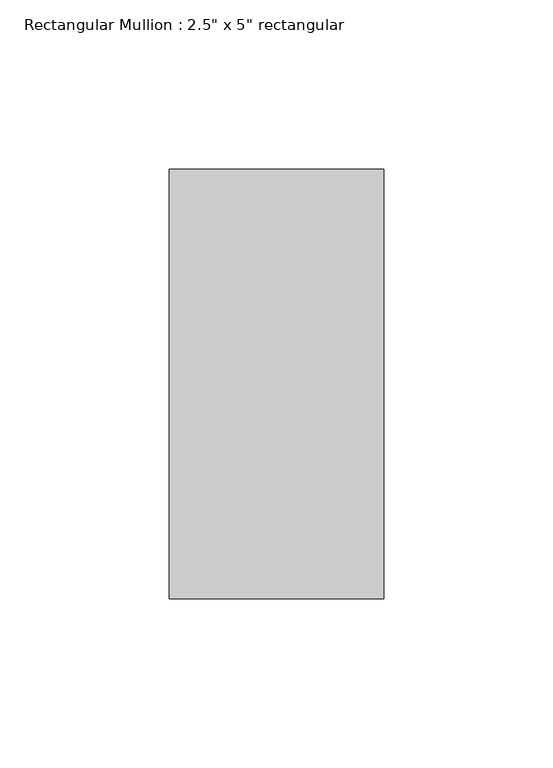
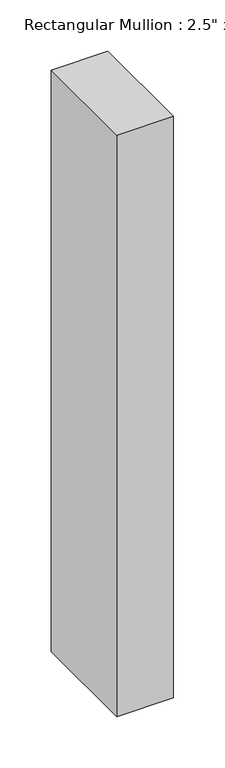
"""IFC4 building model written with IfcOpenShell, lengths in millimetres: member geometry."""

from ifc_helpers import new_model, si_unit, frame, origin, place, context, project, spatial, polyline, outline, extrude, source, transform, mapped, element, save


def member_c769c9ba(model_context):
    return source(origin(), model_context, "Body", "SweptSolid", [
        extrude(outline(polyline([(0.0, 63.5), (0.0, -63.5), (-63.5, -63.5), (-63.5, 63.5), (0.0, 63.5)])), frame((0.0, 0.0, -690.4740338), z_axis=(0.0, 0.0, 1.0), x_axis=(1.0, 0.0, 0.0)), (0.0, 0.0, 1.0), 690.4740338),
    ])


if __name__ == "__main__":
    model = new_model("IFC4")
    model_context = context("Model", 3, world=origin())
    ifc_project = project(units=[si_unit("LENGTHUNIT", "METRE", prefix="MILLI")], contexts=[model_context])
    site = spatial("IfcSite", under=ifc_project)
    building = spatial("IfcBuilding", under=site)
    placement = place(None, origin())
    member_shape = member_c769c9ba(model_context)
    element("IfcMember", 1, ObjectType="Rectangular Mullion : 2.5\" x 5\" rectangular", at=placement, inside=building, context=model_context, shape_type="MappedRepresentation", body=[
        mapped(member_shape, transform((0.0, 0.0, 0.0), x_axis=(1.0, 0.0, 0.0), y_axis=(0.0, 1.0, 0.0), z_axis=(0.0, 0.0, 1.0))),
    ])
    save(model, "model.ifc")

# Revit data of these elements
# Type "Rectangular Mullion : 2.5\" x 5\" rectangular"
#   built-in parameter 1007304 = 0.416667 (stored number, unit not read)
#   built-in parameter 1007301 = 0.104167 (stored number, unit not read)
#   built-in parameter 1007300 = 0.104167 (stored number, unit not read)
# Element 1 (IfcMember, "Rectangular Mullion : 2.5\" x 5\" rectangular")
#   Materials on its faces: "Aluminum"
# Materials
#   "Aluminum": class "Metal", colour RGB 247 247 247, transparency 0, Description = "Aluminum 6061", Cost = 0
